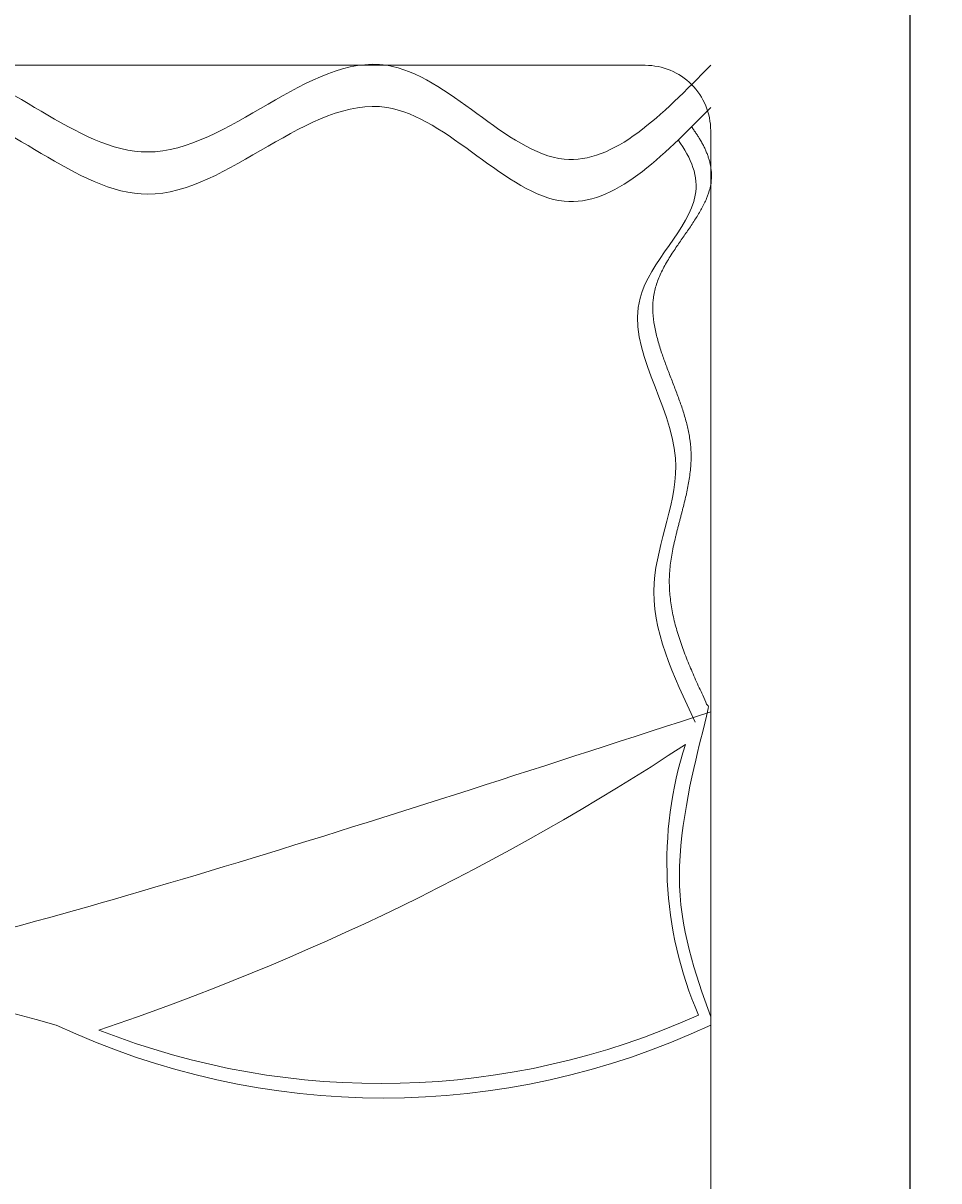
# Model space of a CAD drawing. Units: inches. Extents: x -61 to 1599, y -1316 to 257.
# Tile 121 of 204: x 133 to 181, y 27 to 88. Entities that reach past the tile are written whole.
import ezdxf

# ---------------------------------------------------------------- set-up
doc = ezdxf.new("R2010")
doc.units = ezdxf.units.IN
doc.header["$MEASUREMENT"] = 0
doc.layers.add('A-ANNO-DIMS', color=2, linetype='Continuous', lineweight=18)
doc.layers.add('FURNITURE', color=83, linetype='Continuous', lineweight=18)
doc.styles.get("Standard").update_dxf_attribs({"font": 'arial.ttf'})
doc.dimstyles.get("Standard").update_dxf_attribs({"dimtxt": 0.18, "dimasz": 0.18, "dimexe": 0.18, "dimexo": 0.0625, "dimgap": 0.09, "dimtad": 0, "dimtih": 1, "dimtoh": 1, "dimdec": 0, "dimzin": 0, "dimdsep": 46, "dimlunit": 3, "dimtxsty": 'Standard', "dimcen": 0.09, "dimadec": 0, "dimazin": 0, "dimtfac": 1, "dimtdec": 0, "dimtofl": 0, "dimtmove": 0, "dimatfit": 3, "dimfxl": 1, "dimtolj": 1, "dimtzin": 0, "dimarcsym": 0})

# ---------------------------------------------------------------- blocks, each defined once
blk = doc.blocks.new('BED-DOUBLE')
for points in [[(1.272, 88.537), (1.272, 3.449, 0.414214), (4.722, 0), (66.813, 0, 0.414214), (70.263, 3.449), (70.263, 88.537, 0.414214), (66.813, 91.987), (4.722, 91.987, 0.414214)], [(38.01, 41.126, 0.064396), (68.933, 56.181, 0.181766), (69.614, 41.916, -0.202767)]]:
    blk.add_lwpolyline(points, format="xyb", close=True)
blk.add_lwpolyline([(70.263, 41.387, -0.22309), (35.767, 41.387, 0.142156), (1.272, 41.387)], format="xyb")
for points, knots in [([(70.263, 91.987), (67.707, 89.379), (62.206, 83.764), (52.487, 96.724), (40.92, 82.741), (28.609, 96.737), (15.695, 81.527), (6.205, 88.409), (1.272, 91.987)], [0, 0, 0, 0, 9.176033, 19.753992, 33.150145, 45.209422, 59.881559, 75.764594, 75.764594, 75.764594, 75.764594]), ([(70.263, 89.765), (67.707, 87.157), (62.206, 81.542), (52.487, 94.502), (40.92, 80.519), (28.609, 94.515), (15.695, 79.305), (6.205, 86.187), (1.272, 89.765)], [0, 0, 0, 0, 9.176033, 19.753992, 33.150145, 45.209422, 59.881559, 75.764594, 75.764594, 75.764594, 75.764594]), ([(69.451, 57.362), (68.289, 59.79), (66.113, 64.336), (70.043, 71.905), (64.118, 79.112), (70.314, 84.4), (69.244, 87.088), (68.552, 88.052)], [0, 0, 0, 0, 6.649676, 12.451782, 19.973966, 25.324174, 28.349676, 28.349676, 28.349676, 28.349676])]:
    blk.add_open_spline(points, degree=3, knots=knots)
for points, weights, knots in [([(70.263, 41.825), (68.018, 47.029), (68.018, 52.696), (70.263, 57.9), (69.1, 60.328), (66.924, 64.874), (70.854, 72.444), (64.929, 79.65), (71.186, 84.991), (70.014, 87.727), (69.253, 88.741)], [1, 0.945466318698, 0.945466318698, 1, 1, 1, 1, 1, 1, 1, 1], [0, 0, 0, 0, 0.814571, 0.814571, 0.814571, 7.464247, 13.266353, 20.788537, 26.138745, 29.321895, 29.321895, 29.321895, 29.321895]), ([(70.263, 57.9), (59.862, 50.943), (48.595, 45.5), (36.681, 41.677), (36.463, 41.771), (36.247, 41.868), (36.032, 41.966), (24.597, 45.284), (12.692, 45.258), (1.272, 41.889), (2.723, 44.9), (5.745, 51.172), (0.137, 60.702), (6.828, 69.972), (0.109, 77.787), (4.354, 84.383), (5.398, 86.876)], [1, 0.993520320424, 0.993520320424, 1, 0.99997444972, 0.99997444972, 1, 0.973174868659, 0.973174868659, 1, 1, 1, 1, 1, 1, 1, 1], [0, 0, 0, 0, 0.279074, 0.279074, 0.279074, 0.296584, 0.296584, 0.296584, 0.865868, 0.865868, 0.865868, 9.142578, 18.107734, 25.769226, 34.110801, 40.441511, 40.441511, 40.441511, 40.441511])]:
    blk.add_rational_spline(points, weights, degree=3, knots=knots)
blk = doc.blocks.new('*D687')
at = {"layer": 'A-ANNO-DIMS', "color": 0, "lineweight": -2, "transparency": 16777216}
for p, q in [((289.418, 181.677), (-61.077, 181.677)), ((-60.897, 181.497), (-60.897, -528.952)), ((-60.897, -1239.765), (-60.897, -529.316)), ((319.64, -1239.945), (-61.077, -1239.945))]:
    blk.add_line(p, q, dxfattribs=at)
at = {"layer": 'A-ANNO-DIMS', "color": 0, "transparency": 16777216}
for points in [[(-60.927, 181.497), (-60.867, 181.497), (-60.897, 181.677)], [(-60.927, -1239.765), (-60.867, -1239.765), (-60.897, -1239.945)]]:
    blk.add_solid(points, dxfattribs=at)
at = {"layer": 'DEFPOINTS', "color": 0, "transparency": 16777216}
for p in [(289.481, 181.677), (-60.897, -1239.945), (319.703, -1239.945)]:
    blk.add_point(p, dxfattribs=at)
at = {"layer": 'A-ANNO-DIMS', "color": 0, "transparency": 16777216, "insert": (-60.897, -529.134), "char_height": 0.18, "attachment_point": 5}
blk.add_mtext('\\A1;1421.6', dxfattribs=at)
blk = doc.blocks.new('*D700')
at = {"layer": 'A-ANNO-DIMS', "color": 0, "lineweight": -2, "transparency": 16777216}
for p, q in [((14.703, -616.882), (14.703, 257.457)), ((14.883, 257.277), (96.772, 257.277)), ((179.572, 257.277), (97.683, 257.277)), ((179.752, -616.882), (179.752, 257.457))]:
    blk.add_line(p, q, dxfattribs=at)
at = {"layer": 'A-ANNO-DIMS', "color": 0, "transparency": 16777216}
for points in [[(14.883, 257.307), (14.883, 257.247), (14.703, 257.277)], [(179.572, 257.307), (179.572, 257.247), (179.752, 257.277)]]:
    blk.add_solid(points, dxfattribs=at)
at = {"layer": 'DEFPOINTS', "color": 0, "transparency": 16777216}
for p in [(179.752, 257.277), (14.703, -616.945), (179.752, -616.945)]:
    blk.add_point(p, dxfattribs=at)
at = {"layer": 'A-ANNO-DIMS', "color": 0, "transparency": 16777216, "insert": (97.227, 257.277), "char_height": 0.18, "attachment_point": 5}
blk.add_mtext('\\A1;165.05', dxfattribs=at)

msp = doc.modelspace()

# ---------------------------------------------------------------- block references
at = {"layer": 'FURNITURE'}
msp.add_blockref('BED-DOUBLE', (98.977, -5.797), dxfattribs=at)

# ---------------------------------------------------------------- dimensions: what is measured, and where the dimension line sits
at = {"layer": 'A-ANNO-DIMS'}
dim = msp.add_linear_dim(base=(179.7521, 257.2771), p1=(14.7028, -616.9446), p2=(179.7521, -616.9446), dimstyle='Standard', override={"dimdec": 2, "dimlfac": 1, "dimrnd": 0, "dimzin": 0, "dimdsep": 46, "dimlunit": 2}, dxfattribs=at)
dim.commit()
dim.dimension.update_dxf_attribs({"geometry": '*D700', "text_midpoint": (97.2274, 257.2771)})
dim = msp.add_linear_dim(base=(-60.8972, -1239.9446), p1=(289.4807, 181.6771), p2=(319.7028, -1239.9446), angle=90, dimstyle='Standard', override={"dimdec": 1, "dimlfac": 1, "dimrnd": 0, "dimzin": 0, "dimdsep": 46, "dimlunit": 2}, dxfattribs=at)
dim.commit()
dim.dimension.update_dxf_attribs({"geometry": '*D687', "text_midpoint": (-60.8972, -529.1337)})

doc.saveas('drawing.dxf')
